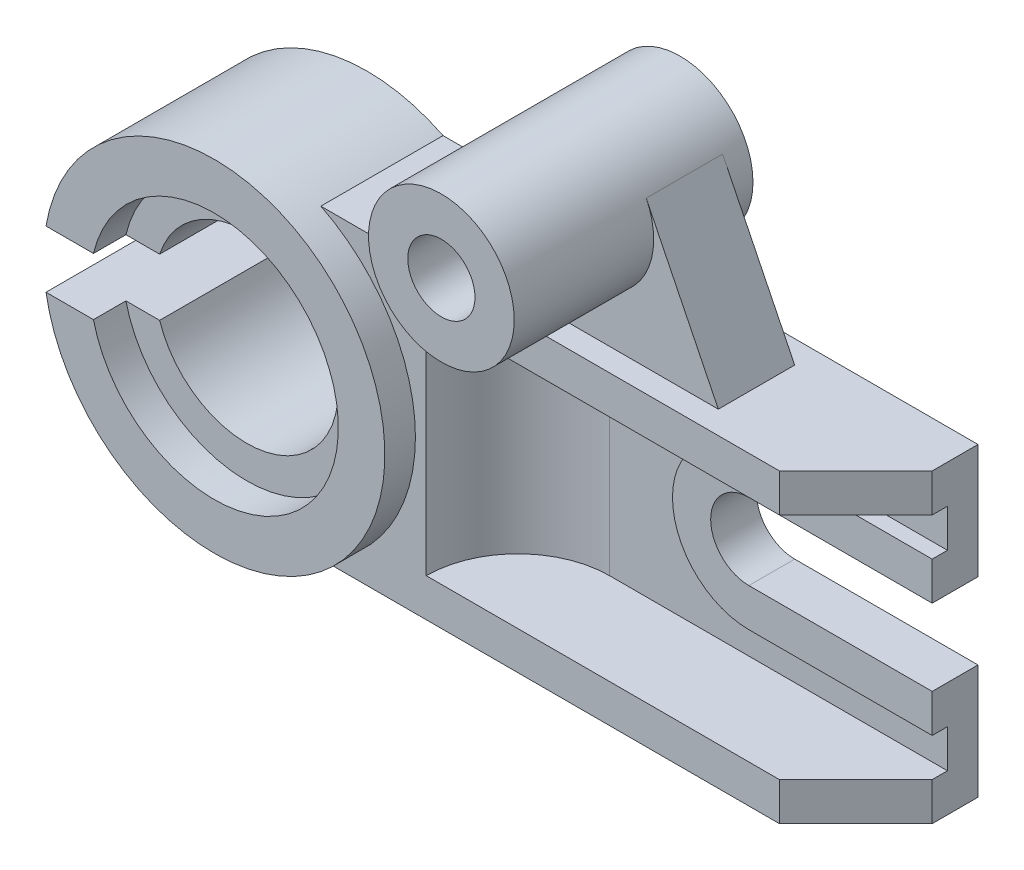
ISO-10303-21;
HEADER;
FILE_DESCRIPTION(('STEP AP214'),'2;1');
FILE_NAME('part.step','',(''),(''),'','','');
FILE_SCHEMA(('AUTOMOTIVE_DESIGN { 1 0 10303 214 1 1 1 1 }'));
ENDSEC;
DATA;
#1=APPLICATION_CONTEXT('core data for automotive mechanical design processes');
#2=APPLICATION_PROTOCOL_DEFINITION('international standard','automotive_design',2000,#1);
#3=PRODUCT_CONTEXT('',#1,'mechanical');
#4=PRODUCT('Part','Part','',(#3));
#5=PRODUCT_RELATED_PRODUCT_CATEGORY('part','',(#4));
#6=PRODUCT_DEFINITION_FORMATION('','',#4);
#7=PRODUCT_DEFINITION_CONTEXT('part definition',#1,'design');
#8=PRODUCT_DEFINITION('design','',#6,#7);
#9=PRODUCT_DEFINITION_SHAPE('','',#8);
#10=(LENGTH_UNIT() NAMED_UNIT(*) SI_UNIT(.MILLI.,.METRE.));
#11=(NAMED_UNIT(*) PLANE_ANGLE_UNIT() SI_UNIT($,.RADIAN.));
#12=(NAMED_UNIT(*) SI_UNIT($,.STERADIAN.) SOLID_ANGLE_UNIT());
#13=UNCERTAINTY_MEASURE_WITH_UNIT(LENGTH_MEASURE(1.E-05),#10,'distance_accuracy_value','');
#14=(GEOMETRIC_REPRESENTATION_CONTEXT(3) GLOBAL_UNCERTAINTY_ASSIGNED_CONTEXT((#13)) GLOBAL_UNIT_ASSIGNED_CONTEXT((#10,
#11,#12)) REPRESENTATION_CONTEXT('',''));
#15=CARTESIAN_POINT('',(0.,0.,0.));
#16=DIRECTION('',(0.,0.,1.));
#17=DIRECTION('',(1.,0.,0.));
#18=AXIS2_PLACEMENT_3D('',#15,#16,#17);
#19=CARTESIAN_POINT('',(4000.,1000.,800.));
#20=DIRECTION('',(-1.,0.,0.));
#21=DIRECTION('',(0.,0.,1.));
#22=AXIS2_PLACEMENT_3D('',#19,#20,#21);
#23=PLANE('',#22);
#24=DIRECTION('',(0.,0.,-1.));
#25=VECTOR('',#24,1.);
#26=CARTESIAN_POINT('',(4000.,1000.,800.));
#27=LINE('',#26,#25);
#28=CARTESIAN_POINT('',(4000.,1000.,299.999999999998));
#29=VERTEX_POINT('',#28);
#30=CARTESIAN_POINT('',(4000.,1000.,0.));
#31=VERTEX_POINT('',#30);
#32=EDGE_CURVE('E361',#29,#31,#27,.T.);
#33=ORIENTED_EDGE('',*,*,#32,.F.);
#34=DIRECTION('',(0.,-1.,0.));
#35=VECTOR('',#34,1.);
#36=CARTESIAN_POINT('',(4000.,750.,299.999999999998));
#37=LINE('',#36,#35);
#38=CARTESIAN_POINT('',(4000.,750.,299.999999999998));
#39=VERTEX_POINT('',#38);
#40=EDGE_CURVE('E430',#29,#39,#37,.T.);
#41=ORIENTED_EDGE('',*,*,#40,.T.);
#42=DIRECTION('',(0.,0.,1.));
#43=VECTOR('',#42,1.);
#44=CARTESIAN_POINT('',(4000.,750.,200.));
#45=LINE('',#44,#43);
#46=CARTESIAN_POINT('',(4000.,750.,200.));
#47=VERTEX_POINT('',#46);
#48=EDGE_CURVE('E335',#47,#39,#45,.T.);
#49=ORIENTED_EDGE('',*,*,#48,.F.);
#50=DIRECTION('',(0.,1.,0.));
#51=VECTOR('',#50,1.);
#52=CARTESIAN_POINT('',(4000.,750.,200.));
#53=LINE('',#52,#51);
#54=CARTESIAN_POINT('',(4000.,500.,200.));
#55=VERTEX_POINT('',#54);
#56=EDGE_CURVE('E320',#55,#47,#53,.T.);
#57=ORIENTED_EDGE('',*,*,#56,.F.);
#58=DIRECTION('',(0.,0.,-1.));
#59=VECTOR('',#58,1.);
#60=CARTESIAN_POINT('',(4000.,500.,300.));
#61=LINE('',#60,#59);
#62=CARTESIAN_POINT('',(4000.,500.,300.));
#63=VERTEX_POINT('',#62);
#64=EDGE_CURVE('E310',#63,#55,#61,.T.);
#65=ORIENTED_EDGE('',*,*,#64,.F.);
#66=DIRECTION('',(0.,1.,0.));
#67=VECTOR('',#66,1.);
#68=CARTESIAN_POINT('',(4000.,500.,300.));
#69=LINE('',#68,#67);
#70=CARTESIAN_POINT('',(4000.,250.,300.));
#71=VERTEX_POINT('',#70);
#72=EDGE_CURVE('E291',#71,#63,#69,.T.);
#73=ORIENTED_EDGE('',*,*,#72,.F.);
#74=DIRECTION('',(0.,0.,1.));
#75=VECTOR('',#74,1.);
#76=CARTESIAN_POINT('',(4000.,250.,0.));
#77=LINE('',#76,#75);
#78=CARTESIAN_POINT('',(4000.,250.,0.));
#79=VERTEX_POINT('',#78);
#80=EDGE_CURVE('E278',#79,#71,#77,.T.);
#81=ORIENTED_EDGE('',*,*,#80,.F.);
#82=DIRECTION('',(0.,1.,0.));
#83=VECTOR('',#82,1.);
#84=CARTESIAN_POINT('',(4000.,1000.,0.));
#85=LINE('',#84,#83);
#86=EDGE_CURVE('E334',#79,#31,#85,.T.);
#87=ORIENTED_EDGE('',*,*,#86,.T.);
#88=EDGE_LOOP('',(#33,#41,#49,#57,#65,#73,#81,#87));
#89=FACE_BOUND('',#88,.T.);
#90=ADVANCED_FACE('F41',(#89),#23,.F.);
#91=CARTESIAN_POINT('',(0.,0.,200.));
#92=DIRECTION('',(0.,0.,1.));
#93=DIRECTION('',(1.,0.,0.));
#94=AXIS2_PLACEMENT_3D('',#91,#92,#93);
#95=PLANE('',#94);
#96=CARTESIAN_POINT('',(4000.,-750.,200.));
#97=VERTEX_POINT('',#96);
#98=CARTESIAN_POINT('',(4000.,-500.,200.));
#99=VERTEX_POINT('',#98);
#100=EDGE_CURVE('E316',#97,#99,#53,.T.);
#101=ORIENTED_EDGE('',*,*,#100,.T.);
#102=DIRECTION('',(1.,0.,0.));
#103=VECTOR('',#102,1.);
#104=CARTESIAN_POINT('',(4000.,-500.,200.));
#105=LINE('',#104,#103);
#106=CARTESIAN_POINT('',(2800.,-500.,200.));
#107=VERTEX_POINT('',#106);
#108=EDGE_CURVE('E305',#107,#99,#105,.T.);
#109=ORIENTED_EDGE('',*,*,#108,.F.);
#110=CARTESIAN_POINT('',(2800.,0.,200.));
#111=DIRECTION('',(0.,0.,1.));
#112=DIRECTION('',(1.,0.,0.));
#113=AXIS2_PLACEMENT_3D('',#110,#111,#112);
#114=CIRCLE('',#113,500.);
#115=CARTESIAN_POINT('',(2800.,500.,200.));
#116=VERTEX_POINT('',#115);
#117=EDGE_CURVE('E276',#116,#107,#114,.T.);
#118=ORIENTED_EDGE('',*,*,#117,.F.);
#119=DIRECTION('',(-1.,0.,0.));
#120=VECTOR('',#119,1.);
#121=CARTESIAN_POINT('',(2800.,500.,200.));
#122=LINE('',#121,#120);
#123=EDGE_CURVE('E293',#55,#116,#122,.T.);
#124=ORIENTED_EDGE('',*,*,#123,.F.);
#125=ORIENTED_EDGE('',*,*,#56,.T.);
#126=DIRECTION('',(-1.,0.,0.));
#127=VECTOR('',#126,1.);
#128=CARTESIAN_POINT('',(1188.,750.,200.));
#129=LINE('',#128,#127);
#130=CARTESIAN_POINT('',(1788.,750.,200.));
#131=VERTEX_POINT('',#130);
#132=EDGE_CURVE('E325',#47,#131,#129,.T.);
#133=ORIENTED_EDGE('',*,*,#132,.T.);
#134=DIRECTION('',(0.,1.,0.));
#135=VECTOR('',#134,1.);
#136=CARTESIAN_POINT('',(1788.,0.,200.));
#137=LINE('',#136,#135);
#138=CARTESIAN_POINT('',(1788.,-750.,200.));
#139=VERTEX_POINT('',#138);
#140=EDGE_CURVE('E415',#131,#139,#137,.F.);
#141=ORIENTED_EDGE('',*,*,#140,.T.);
#142=DIRECTION('',(1.,0.,0.));
#143=VECTOR('',#142,1.);
#144=CARTESIAN_POINT('',(1188.,-750.,200.));
#145=LINE('',#144,#143);
#146=EDGE_CURVE('E314',#139,#97,#145,.T.);
#147=ORIENTED_EDGE('',*,*,#146,.T.);
#148=EDGE_LOOP('',(#101,#109,#118,#124,#125,#133,#141,#147));
#149=FACE_BOUND('',#148,.T.);
#150=ADVANCED_FACE('F501',(#149),#95,.T.);
#151=CARTESIAN_POINT('',(1788.,750.,800.));
#152=DIRECTION('',(0.,1.,0.));
#153=DIRECTION('',(0.,0.,1.));
#154=AXIS2_PLACEMENT_3D('',#151,#152,#153);
#155=CYLINDRICAL_SURFACE('',#154,600.);
#156=DIRECTION('',(0.,-1.,0.));
#157=VECTOR('',#156,1.);
#158=CARTESIAN_POINT('',(1188.,750.,800.));
#159=LINE('',#158,#157);
#160=CARTESIAN_POINT('',(1188.,750.,800.));
#161=VERTEX_POINT('',#160);
#162=CARTESIAN_POINT('',(1188.,-750.,800.));
#163=VERTEX_POINT('',#162);
#164=EDGE_CURVE('E313',#161,#163,#159,.T.);
#165=ORIENTED_EDGE('',*,*,#164,.T.);
#166=CARTESIAN_POINT('',(1788.,-750.,800.));
#167=DIRECTION('',(0.,-1.,0.));
#168=DIRECTION('',(0.,0.,-1.));
#169=AXIS2_PLACEMENT_3D('',#166,#167,#168);
#170=CIRCLE('',#169,600.);
#171=EDGE_CURVE('E416',#139,#163,#170,.F.);
#172=ORIENTED_EDGE('',*,*,#171,.F.);
#173=ORIENTED_EDGE('',*,*,#140,.F.);
#174=CARTESIAN_POINT('',(1788.,750.,800.));
#175=DIRECTION('',(0.,1.,0.));
#176=DIRECTION('',(0.,0.,1.));
#177=AXIS2_PLACEMENT_3D('',#174,#175,#176);
#178=CIRCLE('',#177,600.);
#179=EDGE_CURVE('E419',#161,#131,#178,.F.);
#180=ORIENTED_EDGE('',*,*,#179,.F.);
#181=EDGE_LOOP('',(#165,#172,#173,#180));
#182=FACE_BOUND('',#181,.T.);
#183=ADVANCED_FACE('F458',(#182),#155,.F.);
#184=CARTESIAN_POINT('',(0.,0.,1000.));
#185=DIRECTION('',(0.,0.,-1.));
#186=DIRECTION('',(-1.,0.,0.));
#187=AXIS2_PLACEMENT_3D('',#184,#185,#186);
#188=CYLINDRICAL_SURFACE('',#187,1117.13);
#189=DIRECTION('',(0.,0.,-1.));
#190=VECTOR('',#189,1.);
#191=CARTESIAN_POINT('',(497.975337642338,1000.,800.));
#192=LINE('',#191,#190);
#193=CARTESIAN_POINT('',(497.975337642338,1000.,800.));
#194=VERTEX_POINT('',#193);
#195=CARTESIAN_POINT('',(497.975337642338,1000.,0.));
#196=VERTEX_POINT('',#195);
#197=EDGE_CURVE('E359',#194,#196,#192,.T.);
#198=ORIENTED_EDGE('',*,*,#197,.T.);
#199=CARTESIAN_POINT('',(0.,0.,0.));
#200=DIRECTION('',(0.,0.,1.));
#201=DIRECTION('',(1.,0.,0.));
#202=AXIS2_PLACEMENT_3D('',#199,#200,#201);
#203=CIRCLE('',#202,1117.13);
#204=CARTESIAN_POINT('',(-1101.28251911124,187.5,0.));
#205=VERTEX_POINT('',#204);
#206=EDGE_CURVE('E402',#196,#205,#203,.T.);
#207=ORIENTED_EDGE('',*,*,#206,.T.);
#208=DIRECTION('',(0.,0.,-1.));
#209=VECTOR('',#208,1.);
#210=CARTESIAN_POINT('',(-1101.28251911124,187.5,1000.));
#211=LINE('',#210,#209);
#212=CARTESIAN_POINT('',(-1101.28251911124,187.5,1000.));
#213=VERTEX_POINT('',#212);
#214=EDGE_CURVE('E389',#205,#213,#211,.F.);
#215=ORIENTED_EDGE('',*,*,#214,.T.);
#216=CARTESIAN_POINT('',(0.,0.,1000.));
#217=DIRECTION('',(0.,0.,1.));
#218=DIRECTION('',(1.,0.,0.));
#219=AXIS2_PLACEMENT_3D('',#216,#217,#218);
#220=CIRCLE('',#219,1117.13);
#221=CARTESIAN_POINT('',(-1101.28251911124,-187.5,1000.));
#222=VERTEX_POINT('',#221);
#223=EDGE_CURVE('E404',#222,#213,#220,.T.);
#224=ORIENTED_EDGE('',*,*,#223,.F.);
#225=DIRECTION('',(0.,0.,-1.));
#226=VECTOR('',#225,1.);
#227=CARTESIAN_POINT('',(-1101.28251911124,-187.5,1000.));
#228=LINE('',#227,#226);
#229=CARTESIAN_POINT('',(-1101.28251911124,-187.5,0.));
#230=VERTEX_POINT('',#229);
#231=EDGE_CURVE('E379',#222,#230,#228,.T.);
#232=ORIENTED_EDGE('',*,*,#231,.T.);
#233=CARTESIAN_POINT('',(497.975337642337,-1000.,0.));
#234=VERTEX_POINT('',#233);
#235=EDGE_CURVE('E409',#230,#234,#203,.T.);
#236=ORIENTED_EDGE('',*,*,#235,.T.);
#237=DIRECTION('',(0.,0.,-1.));
#238=VECTOR('',#237,1.);
#239=CARTESIAN_POINT('',(497.975337642338,-1000.,800.));
#240=LINE('',#239,#238);
#241=CARTESIAN_POINT('',(497.975337642338,-1000.,800.));
#242=VERTEX_POINT('',#241);
#243=EDGE_CURVE('E357',#242,#234,#240,.T.);
#244=ORIENTED_EDGE('',*,*,#243,.F.);
#245=CARTESIAN_POINT('',(0.,0.,800.));
#246=DIRECTION('',(0.,0.,-1.));
#247=DIRECTION('',(1.,0.,0.));
#248=AXIS2_PLACEMENT_3D('',#245,#246,#247);
#249=CIRCLE('',#248,1117.13);
#250=EDGE_CURVE('E338',#194,#242,#249,.T.);
#251=ORIENTED_EDGE('',*,*,#250,.F.);
#252=EDGE_LOOP('',(#198,#207,#215,#224,#232,#236,#244,#251));
#253=FACE_BOUND('',#252,.T.);
#254=ADVANCED_FACE('F481',(#253),#188,.T.);
#255=CARTESIAN_POINT('',(0.,0.,1000.));
#256=DIRECTION('',(0.,0.,1.));
#257=DIRECTION('',(1.,0.,0.));
#258=AXIS2_PLACEMENT_3D('',#255,#256,#257);
#259=PLANE('',#258);
#260=DIRECTION('',(-1.,0.,0.));
#261=VECTOR('',#260,1.);
#262=CARTESIAN_POINT('',(-1240.32055513707,187.5,1000.));
#263=LINE('',#262,#261);
#264=CARTESIAN_POINT('',(-790.569415042095,187.5,1000.));
#265=VERTEX_POINT('',#264);
#266=EDGE_CURVE('E369',#265,#213,#263,.T.);
#267=ORIENTED_EDGE('',*,*,#266,.F.);
#268=CARTESIAN_POINT('',(0.,0.,1000.));
#269=DIRECTION('',(0.,0.,1.));
#270=DIRECTION('',(1.,0.,0.));
#271=AXIS2_PLACEMENT_3D('',#268,#269,#270);
#272=CIRCLE('',#271,812.5);
#273=CARTESIAN_POINT('',(-790.569415042095,-187.5,1000.));
#274=VERTEX_POINT('',#273);
#275=EDGE_CURVE('E395',#274,#265,#272,.T.);
#276=ORIENTED_EDGE('',*,*,#275,.F.);
#277=DIRECTION('',(1.,0.,0.));
#278=VECTOR('',#277,1.);
#279=CARTESIAN_POINT('',(-1240.32055513707,-187.5,1000.));
#280=LINE('',#279,#278);
#281=EDGE_CURVE('E362',#222,#274,#280,.T.);
#282=ORIENTED_EDGE('',*,*,#281,.F.);
#283=ORIENTED_EDGE('',*,*,#223,.T.);
#284=EDGE_LOOP('',(#267,#276,#282,#283));
#285=FACE_BOUND('',#284,.T.);
#286=ADVANCED_FACE('F563',(#285),#259,.T.);
#287=CARTESIAN_POINT('',(0.,0.,0.));
#288=DIRECTION('',(0.,0.,1.));
#289=DIRECTION('',(1.,0.,0.));
#290=AXIS2_PLACEMENT_3D('',#287,#288,#289);
#291=PLANE('',#290);
#292=ORIENTED_EDGE('',*,*,#86,.F.);
#293=DIRECTION('',(-1.,0.,0.));
#294=VECTOR('',#293,1.);
#295=CARTESIAN_POINT('',(2800.,250.,0.));
#296=LINE('',#295,#294);
#297=CARTESIAN_POINT('',(2800.,250.,0.));
#298=VERTEX_POINT('',#297);
#299=EDGE_CURVE('E266',#79,#298,#296,.T.);
#300=ORIENTED_EDGE('',*,*,#299,.T.);
#301=CARTESIAN_POINT('',(2800.,0.,0.));
#302=DIRECTION('',(0.,0.,1.));
#303=DIRECTION('',(1.,0.,0.));
#304=AXIS2_PLACEMENT_3D('',#301,#302,#303);
#305=CIRCLE('',#304,250.);
#306=CARTESIAN_POINT('',(2800.,-250.,0.));
#307=VERTEX_POINT('',#306);
#308=EDGE_CURVE('E261',#298,#307,#305,.T.);
#309=ORIENTED_EDGE('',*,*,#308,.T.);
#310=DIRECTION('',(1.,0.,0.));
#311=VECTOR('',#310,1.);
#312=CARTESIAN_POINT('',(4000.,-250.,0.));
#313=LINE('',#312,#311);
#314=CARTESIAN_POINT('',(4000.,-250.,0.));
#315=VERTEX_POINT('',#314);
#316=EDGE_CURVE('E263',#307,#315,#313,.T.);
#317=ORIENTED_EDGE('',*,*,#316,.T.);
#318=CARTESIAN_POINT('',(4000.,-1000.,0.));
#319=VERTEX_POINT('',#318);
#320=EDGE_CURVE('E349',#319,#315,#85,.T.);
#321=ORIENTED_EDGE('',*,*,#320,.F.);
#322=DIRECTION('',(1.,0.,0.));
#323=VECTOR('',#322,1.);
#324=CARTESIAN_POINT('',(497.975337642338,-1000.,0.));
#325=LINE('',#324,#323);
#326=EDGE_CURVE('E342',#234,#319,#325,.T.);
#327=ORIENTED_EDGE('',*,*,#326,.F.);
#328=ORIENTED_EDGE('',*,*,#235,.F.);
#329=DIRECTION('',(1.,0.,0.));
#330=VECTOR('',#329,1.);
#331=CARTESIAN_POINT('',(-1240.32055513707,-187.5,0.));
#332=LINE('',#331,#330);
#333=CARTESIAN_POINT('',(-569.9506557589,-187.5,0.));
#334=VERTEX_POINT('',#333);
#335=EDGE_CURVE('E366',#230,#334,#332,.T.);
#336=ORIENTED_EDGE('',*,*,#335,.T.);
#337=CARTESIAN_POINT('',(0.,0.,0.));
#338=DIRECTION('',(0.,0.,1.));
#339=DIRECTION('',(1.,0.,0.));
#340=AXIS2_PLACEMENT_3D('',#337,#338,#339);
#341=CIRCLE('',#340,600.);
#342=CARTESIAN_POINT('',(-569.9506557589,187.5,0.));
#343=VERTEX_POINT('',#342);
#344=EDGE_CURVE('E392',#334,#343,#341,.T.);
#345=ORIENTED_EDGE('',*,*,#344,.T.);
#346=DIRECTION('',(-1.,0.,0.));
#347=VECTOR('',#346,1.);
#348=CARTESIAN_POINT('',(-1240.32055513707,187.5,0.));
#349=LINE('',#348,#347);
#350=EDGE_CURVE('E367',#343,#205,#349,.T.);
#351=ORIENTED_EDGE('',*,*,#350,.T.);
#352=ORIENTED_EDGE('',*,*,#206,.F.);
#353=DIRECTION('',(-1.,0.,0.));
#354=VECTOR('',#353,1.);
#355=CARTESIAN_POINT('',(497.975337642338,1000.,0.));
#356=LINE('',#355,#354);
#357=EDGE_CURVE('E353',#31,#196,#356,.T.);
#358=ORIENTED_EDGE('',*,*,#357,.F.);
#359=EDGE_LOOP('',(#292,#300,#309,#317,#321,#327,#328,#336,#345,#351,#352,#358));
#360=FACE_BOUND('',#359,.T.);
#361=ADVANCED_FACE('F480',(#360),#291,.F.);
#362=CARTESIAN_POINT('',(0.,0.,787.5));
#363=DIRECTION('',(0.,0.,1.));
#364=DIRECTION('',(1.,0.,0.));
#365=AXIS2_PLACEMENT_3D('',#362,#363,#364);
#366=CYLINDRICAL_SURFACE('',#365,812.5);
#367=ORIENTED_EDGE('',*,*,#275,.T.);
#368=DIRECTION('',(0.,0.,1.));
#369=VECTOR('',#368,1.);
#370=CARTESIAN_POINT('',(-790.569415042095,187.5,787.5));
#371=LINE('',#370,#369);
#372=CARTESIAN_POINT('',(-790.569415042095,187.5,787.5));
#373=VERTEX_POINT('',#372);
#374=EDGE_CURVE('E383',#265,#373,#371,.F.);
#375=ORIENTED_EDGE('',*,*,#374,.T.);
#376=CARTESIAN_POINT('',(0.,0.,787.5));
#377=DIRECTION('',(0.,0.,1.));
#378=DIRECTION('',(1.,0.,0.));
#379=AXIS2_PLACEMENT_3D('',#376,#377,#378);
#380=CIRCLE('',#379,812.5);
#381=CARTESIAN_POINT('',(-790.569415042095,-187.5,787.5));
#382=VERTEX_POINT('',#381);
#383=EDGE_CURVE('E396',#382,#373,#380,.T.);
#384=ORIENTED_EDGE('',*,*,#383,.F.);
#385=DIRECTION('',(0.,0.,1.));
#386=VECTOR('',#385,1.);
#387=CARTESIAN_POINT('',(-790.569415042095,-187.5,787.5));
#388=LINE('',#387,#386);
#389=EDGE_CURVE('E380',#382,#274,#388,.T.);
#390=ORIENTED_EDGE('',*,*,#389,.T.);
#391=EDGE_LOOP('',(#367,#375,#384,#390));
#392=FACE_BOUND('',#391,.T.);
#393=ADVANCED_FACE('F556',(#392),#366,.F.);
#394=CARTESIAN_POINT('',(0.,0.,787.5));
#395=DIRECTION('',(0.,0.,1.));
#396=DIRECTION('',(1.,0.,0.));
#397=AXIS2_PLACEMENT_3D('',#394,#395,#396);
#398=PLANE('',#397);
#399=DIRECTION('',(-1.,0.,0.));
#400=VECTOR('',#399,1.);
#401=CARTESIAN_POINT('',(0.,187.5,787.5));
#402=LINE('',#401,#400);
#403=CARTESIAN_POINT('',(-569.9506557589,187.5,787.5));
#404=VERTEX_POINT('',#403);
#405=EDGE_CURVE('E384',#404,#373,#402,.T.);
#406=ORIENTED_EDGE('',*,*,#405,.F.);
#407=CARTESIAN_POINT('',(0.,0.,787.5));
#408=DIRECTION('',(0.,0.,1.));
#409=DIRECTION('',(1.,0.,0.));
#410=AXIS2_PLACEMENT_3D('',#407,#408,#409);
#411=CIRCLE('',#410,600.);
#412=CARTESIAN_POINT('',(-569.9506557589,-187.5,787.5));
#413=VERTEX_POINT('',#412);
#414=EDGE_CURVE('E391',#413,#404,#411,.T.);
#415=ORIENTED_EDGE('',*,*,#414,.F.);
#416=DIRECTION('',(1.,0.,0.));
#417=VECTOR('',#416,1.);
#418=CARTESIAN_POINT('',(0.,-187.5,787.5));
#419=LINE('',#418,#417);
#420=EDGE_CURVE('E373',#382,#413,#419,.T.);
#421=ORIENTED_EDGE('',*,*,#420,.F.);
#422=ORIENTED_EDGE('',*,*,#383,.T.);
#423=EDGE_LOOP('',(#406,#415,#421,#422));
#424=FACE_BOUND('',#423,.T.);
#425=ADVANCED_FACE('F555',(#424),#398,.T.);
#426=CARTESIAN_POINT('',(0.,0.,0.));
#427=DIRECTION('',(0.,0.,1.));
#428=DIRECTION('',(1.,0.,0.));
#429=AXIS2_PLACEMENT_3D('',#426,#427,#428);
#430=CYLINDRICAL_SURFACE('',#429,600.);
#431=ORIENTED_EDGE('',*,*,#414,.T.);
#432=DIRECTION('',(0.,0.,1.));
#433=VECTOR('',#432,1.);
#434=CARTESIAN_POINT('',(-569.9506557589,187.5,0.));
#435=LINE('',#434,#433);
#436=EDGE_CURVE('E412',#404,#343,#435,.F.);
#437=ORIENTED_EDGE('',*,*,#436,.T.);
#438=ORIENTED_EDGE('',*,*,#344,.F.);
#439=DIRECTION('',(0.,0.,1.));
#440=VECTOR('',#439,1.);
#441=CARTESIAN_POINT('',(-569.9506557589,-187.5,0.));
#442=LINE('',#441,#440);
#443=EDGE_CURVE('E410',#334,#413,#442,.T.);
#444=ORIENTED_EDGE('',*,*,#443,.T.);
#445=EDGE_LOOP('',(#431,#437,#438,#444));
#446=FACE_BOUND('',#445,.T.);
#447=ADVANCED_FACE('F546',(#446),#430,.F.);
#448=CARTESIAN_POINT('',(-1240.32055513707,-187.5,0.));
#449=DIRECTION('',(0.,-1.,0.));
#450=DIRECTION('',(0.,0.,-1.));
#451=AXIS2_PLACEMENT_3D('',#448,#449,#450);
#452=PLANE('',#451);
#453=ORIENTED_EDGE('',*,*,#281,.T.);
#454=ORIENTED_EDGE('',*,*,#389,.F.);
#455=ORIENTED_EDGE('',*,*,#420,.T.);
#456=ORIENTED_EDGE('',*,*,#443,.F.);
#457=ORIENTED_EDGE('',*,*,#335,.F.);
#458=ORIENTED_EDGE('',*,*,#231,.F.);
#459=EDGE_LOOP('',(#453,#454,#455,#456,#457,#458));
#460=FACE_BOUND('',#459,.T.);
#461=ADVANCED_FACE('F542',(#460),#452,.F.);
#462=CARTESIAN_POINT('',(-1240.32055513707,187.5,0.));
#463=DIRECTION('',(0.,1.,0.));
#464=DIRECTION('',(0.,0.,1.));
#465=AXIS2_PLACEMENT_3D('',#462,#463,#464);
#466=PLANE('',#465);
#467=ORIENTED_EDGE('',*,*,#350,.F.);
#468=ORIENTED_EDGE('',*,*,#436,.F.);
#469=ORIENTED_EDGE('',*,*,#405,.T.);
#470=ORIENTED_EDGE('',*,*,#374,.F.);
#471=ORIENTED_EDGE('',*,*,#266,.T.);
#472=ORIENTED_EDGE('',*,*,#214,.F.);
#473=EDGE_LOOP('',(#467,#468,#469,#470,#471,#472));
#474=FACE_BOUND('',#473,.T.);
#475=ADVANCED_FACE('F537',(#474),#466,.F.);
#476=DIRECTION('',(0.,0.,1.));
#477=VECTOR('',#476,1.);
#478=CARTESIAN_POINT('',(4000.,-750.,200.));
#479=LINE('',#478,#477);
#480=CARTESIAN_POINT('',(4000.,-750.,299.999999999998));
#481=VERTEX_POINT('',#480);
#482=EDGE_CURVE('E323',#97,#481,#479,.T.);
#483=ORIENTED_EDGE('',*,*,#482,.T.);
#484=DIRECTION('',(0.,-1.,0.));
#485=VECTOR('',#484,1.);
#486=CARTESIAN_POINT('',(4000.,-1000.,299.999999999998));
#487=LINE('',#486,#485);
#488=CARTESIAN_POINT('',(4000.,-1000.,299.999999999998));
#489=VERTEX_POINT('',#488);
#490=EDGE_CURVE('E49',#481,#489,#487,.T.);
#491=ORIENTED_EDGE('',*,*,#490,.T.);
#492=DIRECTION('',(0.,0.,-1.));
#493=VECTOR('',#492,1.);
#494=CARTESIAN_POINT('',(4000.,-1000.,800.));
#495=LINE('',#494,#493);
#496=EDGE_CURVE('E347',#489,#319,#495,.T.);
#497=ORIENTED_EDGE('',*,*,#496,.T.);
#498=ORIENTED_EDGE('',*,*,#320,.T.);
#499=DIRECTION('',(0.,0.,1.));
#500=VECTOR('',#499,1.);
#501=CARTESIAN_POINT('',(4000.,-250.,0.));
#502=LINE('',#501,#500);
#503=CARTESIAN_POINT('',(4000.,-250.,300.));
#504=VERTEX_POINT('',#503);
#505=EDGE_CURVE('E282',#315,#504,#502,.T.);
#506=ORIENTED_EDGE('',*,*,#505,.T.);
#507=CARTESIAN_POINT('',(4000.,-500.,300.));
#508=VERTEX_POINT('',#507);
#509=EDGE_CURVE('E295',#508,#504,#69,.T.);
#510=ORIENTED_EDGE('',*,*,#509,.F.);
#511=DIRECTION('',(0.,0.,-1.));
#512=VECTOR('',#511,1.);
#513=CARTESIAN_POINT('',(4000.,-500.,300.));
#514=LINE('',#513,#512);
#515=EDGE_CURVE('E307',#508,#99,#514,.T.);
#516=ORIENTED_EDGE('',*,*,#515,.T.);
#517=ORIENTED_EDGE('',*,*,#100,.F.);
#518=EDGE_LOOP('',(#483,#491,#497,#498,#506,#510,#516,#517));
#519=FACE_BOUND('',#518,.T.);
#520=ADVANCED_FACE('F438',(#519),#23,.F.);
#521=CARTESIAN_POINT('',(497.975337642338,1000.,800.));
#522=DIRECTION('',(0.,-1.,0.));
#523=DIRECTION('',(1.,0.,0.));
#524=AXIS2_PLACEMENT_3D('',#521,#522,#523);
#525=PLANE('',#524);
#526=DIRECTION('',(0.,0.,-1.));
#527=VECTOR('',#526,1.);
#528=CARTESIAN_POINT('',(2950.,1000.,650.));
#529=LINE('',#528,#527);
#530=CARTESIAN_POINT('',(2950.,1000.,650.));
#531=VERTEX_POINT('',#530);
#532=CARTESIAN_POINT('',(2950.,1000.,150.));
#533=VERTEX_POINT('',#532);
#534=EDGE_CURVE('E60',#531,#533,#529,.T.);
#535=ORIENTED_EDGE('',*,*,#534,.F.);
#536=DIRECTION('',(1.,0.,0.));
#537=VECTOR('',#536,1.);
#538=CARTESIAN_POINT('',(1150.,1000.,650.));
#539=LINE('',#538,#537);
#540=CARTESIAN_POINT('',(1150.,1000.,650.));
#541=VERTEX_POINT('',#540);
#542=EDGE_CURVE('E62',#541,#531,#539,.T.);
#543=ORIENTED_EDGE('',*,*,#542,.F.);
#544=DIRECTION('',(0.,0.,-1.));
#545=VECTOR('',#544,1.);
#546=CARTESIAN_POINT('',(1150.,1000.,650.));
#547=LINE('',#546,#545);
#548=CARTESIAN_POINT('',(1150.,1000.,150.));
#549=VERTEX_POINT('',#548);
#550=EDGE_CURVE('E243',#541,#549,#547,.T.);
#551=ORIENTED_EDGE('',*,*,#550,.T.);
#552=DIRECTION('',(1.,0.,0.));
#553=VECTOR('',#552,1.);
#554=CARTESIAN_POINT('',(1150.,1000.,150.));
#555=LINE('',#554,#553);
#556=EDGE_CURVE('E233',#549,#533,#555,.T.);
#557=ORIENTED_EDGE('',*,*,#556,.T.);
#558=EDGE_LOOP('',(#535,#543,#551,#557));
#559=FACE_BOUND('',#558,.T.);
#560=DIRECTION('',(-1.,0.,0.));
#561=VECTOR('',#560,1.);
#562=CARTESIAN_POINT('',(497.975337642338,1000.,800.));
#563=LINE('',#562,#561);
#564=CARTESIAN_POINT('',(3500.,1000.,800.));
#565=VERTEX_POINT('',#564);
#566=EDGE_CURVE('E336',#565,#194,#563,.T.);
#567=ORIENTED_EDGE('',*,*,#566,.F.);
#568=DIRECTION('',(0.707106781186546,0.,-0.707106781186549));
#569=VECTOR('',#568,1.);
#570=CARTESIAN_POINT('',(3500.,1000.,800.));
#571=LINE('',#570,#569);
#572=EDGE_CURVE('E424',#565,#29,#571,.T.);
#573=ORIENTED_EDGE('',*,*,#572,.T.);
#574=ORIENTED_EDGE('',*,*,#32,.T.);
#575=ORIENTED_EDGE('',*,*,#357,.T.);
#576=ORIENTED_EDGE('',*,*,#197,.F.);
#577=EDGE_LOOP('',(#567,#573,#574,#575,#576));
#578=FACE_BOUND('',#577,.T.);
#579=ADVANCED_FACE('F468',(#559,#578),#525,.F.);
#580=CARTESIAN_POINT('',(497.975337642338,-1000.,800.));
#581=DIRECTION('',(0.,1.,0.));
#582=DIRECTION('',(0.,0.,1.));
#583=AXIS2_PLACEMENT_3D('',#580,#581,#582);
#584=PLANE('',#583);
#585=ORIENTED_EDGE('',*,*,#496,.F.);
#586=DIRECTION('',(-0.707106781186546,0.,0.707106781186549));
#587=VECTOR('',#586,1.);
#588=CARTESIAN_POINT('',(3500.,-1000.,800.));
#589=LINE('',#588,#587);
#590=CARTESIAN_POINT('',(3500.,-1000.,800.));
#591=VERTEX_POINT('',#590);
#592=EDGE_CURVE('E11',#489,#591,#589,.T.);
#593=ORIENTED_EDGE('',*,*,#592,.T.);
#594=DIRECTION('',(1.,0.,0.));
#595=VECTOR('',#594,1.);
#596=CARTESIAN_POINT('',(497.975337642338,-1000.,800.));
#597=LINE('',#596,#595);
#598=EDGE_CURVE('E341',#242,#591,#597,.T.);
#599=ORIENTED_EDGE('',*,*,#598,.F.);
#600=ORIENTED_EDGE('',*,*,#243,.T.);
#601=ORIENTED_EDGE('',*,*,#326,.T.);
#602=EDGE_LOOP('',(#585,#593,#599,#600,#601));
#603=FACE_BOUND('',#602,.T.);
#604=ADVANCED_FACE('F443',(#603),#584,.F.);
#605=CARTESIAN_POINT('',(0.,0.,800.));
#606=DIRECTION('',(0.,0.,1.));
#607=DIRECTION('',(1.,0.,0.));
#608=AXIS2_PLACEMENT_3D('',#605,#606,#607);
#609=PLANE('',#608);
#610=ORIENTED_EDGE('',*,*,#598,.T.);
#611=DIRECTION('',(0.,1.,0.));
#612=VECTOR('',#611,1.);
#613=CARTESIAN_POINT('',(3500.,-750.,800.));
#614=LINE('',#613,#612);
#615=CARTESIAN_POINT('',(3500.,-750.,800.));
#616=VERTEX_POINT('',#615);
#617=EDGE_CURVE('E431',#591,#616,#614,.T.);
#618=ORIENTED_EDGE('',*,*,#617,.T.);
#619=DIRECTION('',(1.,0.,0.));
#620=VECTOR('',#619,1.);
#621=CARTESIAN_POINT('',(1188.,-750.,800.));
#622=LINE('',#621,#620);
#623=EDGE_CURVE('E329',#163,#616,#622,.T.);
#624=ORIENTED_EDGE('',*,*,#623,.F.);
#625=ORIENTED_EDGE('',*,*,#164,.F.);
#626=DIRECTION('',(-1.,0.,0.));
#627=VECTOR('',#626,1.);
#628=CARTESIAN_POINT('',(1188.,750.,800.));
#629=LINE('',#628,#627);
#630=CARTESIAN_POINT('',(3500.,750.,800.));
#631=VERTEX_POINT('',#630);
#632=EDGE_CURVE('E319',#631,#161,#629,.T.);
#633=ORIENTED_EDGE('',*,*,#632,.F.);
#634=DIRECTION('',(0.,1.,0.));
#635=VECTOR('',#634,1.);
#636=CARTESIAN_POINT('',(3500.,1000.,800.));
#637=LINE('',#636,#635);
#638=EDGE_CURVE('E422',#631,#565,#637,.T.);
#639=ORIENTED_EDGE('',*,*,#638,.T.);
#640=ORIENTED_EDGE('',*,*,#566,.T.);
#641=ORIENTED_EDGE('',*,*,#250,.T.);
#642=EDGE_LOOP('',(#610,#618,#624,#625,#633,#639,#640,#641));
#643=FACE_BOUND('',#642,.T.);
#644=ADVANCED_FACE('F452',(#643),#609,.T.);
#645=CARTESIAN_POINT('',(1188.,750.,200.));
#646=DIRECTION('',(0.,1.,0.));
#647=DIRECTION('',(0.,0.,1.));
#648=AXIS2_PLACEMENT_3D('',#645,#646,#647);
#649=PLANE('',#648);
#650=ORIENTED_EDGE('',*,*,#48,.T.);
#651=DIRECTION('',(-0.707106781186546,0.,0.707106781186549));
#652=VECTOR('',#651,1.);
#653=CARTESIAN_POINT('',(3500.,750.,800.));
#654=LINE('',#653,#652);
#655=EDGE_CURVE('E429',#39,#631,#654,.T.);
#656=ORIENTED_EDGE('',*,*,#655,.T.);
#657=ORIENTED_EDGE('',*,*,#632,.T.);
#658=ORIENTED_EDGE('',*,*,#179,.T.);
#659=ORIENTED_EDGE('',*,*,#132,.F.);
#660=EDGE_LOOP('',(#650,#656,#657,#658,#659));
#661=FACE_BOUND('',#660,.T.);
#662=ADVANCED_FACE('F506',(#661),#649,.F.);
#663=CARTESIAN_POINT('',(1188.,-750.,200.));
#664=DIRECTION('',(0.,-1.,0.));
#665=DIRECTION('',(0.,0.,-1.));
#666=AXIS2_PLACEMENT_3D('',#663,#664,#665);
#667=PLANE('',#666);
#668=ORIENTED_EDGE('',*,*,#623,.T.);
#669=DIRECTION('',(0.707106781186546,0.,-0.707106781186549));
#670=VECTOR('',#669,1.);
#671=CARTESIAN_POINT('',(3500.,-750.,800.));
#672=LINE('',#671,#670);
#673=EDGE_CURVE('E432',#616,#481,#672,.T.);
#674=ORIENTED_EDGE('',*,*,#673,.T.);
#675=ORIENTED_EDGE('',*,*,#482,.F.);
#676=ORIENTED_EDGE('',*,*,#146,.F.);
#677=ORIENTED_EDGE('',*,*,#171,.T.);
#678=EDGE_LOOP('',(#668,#674,#675,#676,#677));
#679=FACE_BOUND('',#678,.T.);
#680=ADVANCED_FACE('F451',(#679),#667,.F.);
#681=CARTESIAN_POINT('',(2800.,0.,300.));
#682=DIRECTION('',(0.,0.,-1.));
#683=DIRECTION('',(-1.,0.,0.));
#684=AXIS2_PLACEMENT_3D('',#681,#682,#683);
#685=CYLINDRICAL_SURFACE('',#684,500.);
#686=ORIENTED_EDGE('',*,*,#117,.T.);
#687=DIRECTION('',(0.,0.,-1.));
#688=VECTOR('',#687,1.);
#689=CARTESIAN_POINT('',(2800.,-500.,300.));
#690=LINE('',#689,#688);
#691=CARTESIAN_POINT('',(2800.,-500.,300.));
#692=VERTEX_POINT('',#691);
#693=EDGE_CURVE('E315',#692,#107,#690,.T.);
#694=ORIENTED_EDGE('',*,*,#693,.F.);
#695=CARTESIAN_POINT('',(2800.,0.,300.));
#696=DIRECTION('',(0.,0.,1.));
#697=DIRECTION('',(1.,0.,0.));
#698=AXIS2_PLACEMENT_3D('',#695,#696,#697);
#699=CIRCLE('',#698,500.);
#700=CARTESIAN_POINT('',(2800.,500.,300.));
#701=VERTEX_POINT('',#700);
#702=EDGE_CURVE('E290',#701,#692,#699,.T.);
#703=ORIENTED_EDGE('',*,*,#702,.F.);
#704=DIRECTION('',(0.,0.,-1.));
#705=VECTOR('',#704,1.);
#706=CARTESIAN_POINT('',(2800.,500.,300.));
#707=LINE('',#706,#705);
#708=EDGE_CURVE('E299',#701,#116,#707,.T.);
#709=ORIENTED_EDGE('',*,*,#708,.T.);
#710=EDGE_LOOP('',(#686,#694,#703,#709));
#711=FACE_BOUND('',#710,.T.);
#712=ADVANCED_FACE('F590',(#711),#685,.T.);
#713=CARTESIAN_POINT('',(4000.,-500.,300.));
#714=DIRECTION('',(0.,1.,0.));
#715=DIRECTION('',(0.,0.,1.));
#716=AXIS2_PLACEMENT_3D('',#713,#714,#715);
#717=PLANE('',#716);
#718=ORIENTED_EDGE('',*,*,#108,.T.);
#719=ORIENTED_EDGE('',*,*,#515,.F.);
#720=DIRECTION('',(1.,0.,0.));
#721=VECTOR('',#720,1.);
#722=CARTESIAN_POINT('',(4000.,-500.,300.));
#723=LINE('',#722,#721);
#724=EDGE_CURVE('E289',#692,#508,#723,.T.);
#725=ORIENTED_EDGE('',*,*,#724,.F.);
#726=ORIENTED_EDGE('',*,*,#693,.T.);
#727=EDGE_LOOP('',(#718,#719,#725,#726));
#728=FACE_BOUND('',#727,.T.);
#729=ADVANCED_FACE('F498',(#728),#717,.F.);
#730=CARTESIAN_POINT('',(2800.,500.,300.));
#731=DIRECTION('',(0.,-1.,0.));
#732=DIRECTION('',(1.,0.,0.));
#733=AXIS2_PLACEMENT_3D('',#730,#731,#732);
#734=PLANE('',#733);
#735=ORIENTED_EDGE('',*,*,#123,.T.);
#736=ORIENTED_EDGE('',*,*,#708,.F.);
#737=DIRECTION('',(-1.,0.,0.));
#738=VECTOR('',#737,1.);
#739=CARTESIAN_POINT('',(2800.,500.,300.));
#740=LINE('',#739,#738);
#741=EDGE_CURVE('E300',#63,#701,#740,.T.);
#742=ORIENTED_EDGE('',*,*,#741,.F.);
#743=ORIENTED_EDGE('',*,*,#64,.T.);
#744=EDGE_LOOP('',(#735,#736,#742,#743));
#745=FACE_BOUND('',#744,.T.);
#746=ADVANCED_FACE('F512',(#745),#734,.F.);
#747=CARTESIAN_POINT('',(2800.,0.,300.));
#748=DIRECTION('',(0.,0.,1.));
#749=DIRECTION('',(1.,0.,0.));
#750=AXIS2_PLACEMENT_3D('',#747,#748,#749);
#751=PLANE('',#750);
#752=DIRECTION('',(-1.,0.,0.));
#753=VECTOR('',#752,1.);
#754=CARTESIAN_POINT('',(2800.,250.,300.));
#755=LINE('',#754,#753);
#756=CARTESIAN_POINT('',(2800.,250.,300.));
#757=VERTEX_POINT('',#756);
#758=EDGE_CURVE('E265',#71,#757,#755,.T.);
#759=ORIENTED_EDGE('',*,*,#758,.F.);
#760=ORIENTED_EDGE('',*,*,#72,.T.);
#761=ORIENTED_EDGE('',*,*,#741,.T.);
#762=ORIENTED_EDGE('',*,*,#702,.T.);
#763=ORIENTED_EDGE('',*,*,#724,.T.);
#764=ORIENTED_EDGE('',*,*,#509,.T.);
#765=DIRECTION('',(1.,0.,0.));
#766=VECTOR('',#765,1.);
#767=CARTESIAN_POINT('',(4000.,-250.,300.));
#768=LINE('',#767,#766);
#769=CARTESIAN_POINT('',(2800.,-250.,300.));
#770=VERTEX_POINT('',#769);
#771=EDGE_CURVE('E271',#770,#504,#768,.T.);
#772=ORIENTED_EDGE('',*,*,#771,.F.);
#773=CARTESIAN_POINT('',(2800.,0.,300.));
#774=DIRECTION('',(0.,0.,1.));
#775=DIRECTION('',(1.,0.,0.));
#776=AXIS2_PLACEMENT_3D('',#773,#774,#775);
#777=CIRCLE('',#776,250.);
#778=EDGE_CURVE('E258',#757,#770,#777,.T.);
#779=ORIENTED_EDGE('',*,*,#778,.F.);
#780=EDGE_LOOP('',(#759,#760,#761,#762,#763,#764,#772,#779));
#781=FACE_BOUND('',#780,.T.);
#782=ADVANCED_FACE('F495',(#781),#751,.T.);
#783=CARTESIAN_POINT('',(2800.,0.,0.));
#784=DIRECTION('',(0.,0.,1.));
#785=DIRECTION('',(1.,0.,0.));
#786=AXIS2_PLACEMENT_3D('',#783,#784,#785);
#787=CYLINDRICAL_SURFACE('',#786,250.);
#788=ORIENTED_EDGE('',*,*,#778,.T.);
#789=DIRECTION('',(0.,0.,1.));
#790=VECTOR('',#789,1.);
#791=CARTESIAN_POINT('',(2800.,-250.,0.));
#792=LINE('',#791,#790);
#793=EDGE_CURVE('E272',#307,#770,#792,.T.);
#794=ORIENTED_EDGE('',*,*,#793,.F.);
#795=ORIENTED_EDGE('',*,*,#308,.F.);
#796=DIRECTION('',(0.,0.,1.));
#797=VECTOR('',#796,1.);
#798=CARTESIAN_POINT('',(2800.,250.,0.));
#799=LINE('',#798,#797);
#800=EDGE_CURVE('E280',#298,#757,#799,.T.);
#801=ORIENTED_EDGE('',*,*,#800,.T.);
#802=EDGE_LOOP('',(#788,#794,#795,#801));
#803=FACE_BOUND('',#802,.T.);
#804=ADVANCED_FACE('F517',(#803),#787,.F.);
#805=CARTESIAN_POINT('',(2800.,250.,0.));
#806=DIRECTION('',(0.,1.,0.));
#807=DIRECTION('',(-1.,0.,0.));
#808=AXIS2_PLACEMENT_3D('',#805,#806,#807);
#809=PLANE('',#808);
#810=ORIENTED_EDGE('',*,*,#758,.T.);
#811=ORIENTED_EDGE('',*,*,#800,.F.);
#812=ORIENTED_EDGE('',*,*,#299,.F.);
#813=ORIENTED_EDGE('',*,*,#80,.T.);
#814=EDGE_LOOP('',(#810,#811,#812,#813));
#815=FACE_BOUND('',#814,.T.);
#816=ADVANCED_FACE('F514',(#815),#809,.F.);
#817=CARTESIAN_POINT('',(4000.,-250.,0.));
#818=DIRECTION('',(0.,-1.,0.));
#819=DIRECTION('',(0.,0.,-1.));
#820=AXIS2_PLACEMENT_3D('',#817,#818,#819);
#821=PLANE('',#820);
#822=ORIENTED_EDGE('',*,*,#771,.T.);
#823=ORIENTED_EDGE('',*,*,#505,.F.);
#824=ORIENTED_EDGE('',*,*,#316,.F.);
#825=ORIENTED_EDGE('',*,*,#793,.T.);
#826=EDGE_LOOP('',(#822,#823,#824,#825));
#827=FACE_BOUND('',#826,.T.);
#828=ADVANCED_FACE('F520',(#827),#821,.F.);
#829=CARTESIAN_POINT('',(3500.,0.,800.));
#830=DIRECTION('',(0.707106781186549,0.,0.707106781186546));
#831=DIRECTION('',(0.,-1.,0.));
#832=AXIS2_PLACEMENT_3D('',#829,#830,#831);
#833=PLANE('',#832);
#834=ORIENTED_EDGE('',*,*,#655,.F.);
#835=ORIENTED_EDGE('',*,*,#40,.F.);
#836=ORIENTED_EDGE('',*,*,#572,.F.);
#837=ORIENTED_EDGE('',*,*,#638,.F.);
#838=EDGE_LOOP('',(#834,#835,#836,#837));
#839=FACE_BOUND('',#838,.T.);
#840=ADVANCED_FACE('F467',(#839),#833,.T.);
#841=CARTESIAN_POINT('',(3500.,0.,800.));
#842=DIRECTION('',(0.707106781186549,0.,0.707106781186546));
#843=DIRECTION('',(0.,-1.,0.));
#844=AXIS2_PLACEMENT_3D('',#841,#842,#843);
#845=PLANE('',#844);
#846=ORIENTED_EDGE('',*,*,#592,.F.);
#847=ORIENTED_EDGE('',*,*,#490,.F.);
#848=ORIENTED_EDGE('',*,*,#673,.F.);
#849=ORIENTED_EDGE('',*,*,#617,.F.);
#850=EDGE_LOOP('',(#846,#847,#848,#849));
#851=FACE_BOUND('',#850,.T.);
#852=ADVANCED_FACE('F42',(#851),#845,.T.);
#853=CARTESIAN_POINT('',(2950.,1000.,650.));
#854=DIRECTION('',(-0.897461190076744,-0.441093428092093,0.));
#855=DIRECTION('',(0.441093428092093,-0.897461190076744,0.));
#856=AXIS2_PLACEMENT_3D('',#853,#854,#855);
#857=PLANE('',#856);
#858=DIRECTION('',(-0.441093428092093,0.897461190076744,0.));
#859=VECTOR('',#858,1.);
#860=CARTESIAN_POINT('',(2950.,1000.,150.));
#861=LINE('',#860,#859);
#862=CARTESIAN_POINT('',(2477.99475424165,1960.35525038998,150.));
#863=VERTEX_POINT('',#862);
#864=EDGE_CURVE('E248',#533,#863,#861,.T.);
#865=ORIENTED_EDGE('',*,*,#864,.T.);
#866=DIRECTION('',(0.,0.,-1.));
#867=VECTOR('',#866,1.);
#868=CARTESIAN_POINT('',(2477.99475424165,1960.35525038998,650.));
#869=LINE('',#868,#867);
#870=CARTESIAN_POINT('',(2477.99475424165,1960.35525038998,650.));
#871=VERTEX_POINT('',#870);
#872=EDGE_CURVE('E245',#871,#863,#869,.T.);
#873=ORIENTED_EDGE('',*,*,#872,.F.);
#874=DIRECTION('',(-0.441093428092093,0.897461190076744,0.));
#875=VECTOR('',#874,1.);
#876=CARTESIAN_POINT('',(2950.,1000.,650.));
#877=LINE('',#876,#875);
#878=EDGE_CURVE('E257',#531,#871,#877,.T.);
#879=ORIENTED_EDGE('',*,*,#878,.F.);
#880=ORIENTED_EDGE('',*,*,#534,.T.);
#881=EDGE_LOOP('',(#865,#873,#879,#880));
#882=FACE_BOUND('',#881,.T.);
#883=ADVANCED_FACE('F655',(#882),#857,.F.);
#884=CARTESIAN_POINT('',(1150.,1000.,650.));
#885=DIRECTION('',(0.897461190076744,-0.441093428092092,0.));
#886=DIRECTION('',(0.441093428092092,0.897461190076744,0.));
#887=AXIS2_PLACEMENT_3D('',#884,#885,#886);
#888=PLANE('',#887);
#889=DIRECTION('',(-0.441093428092092,-0.897461190076744,0.));
#890=VECTOR('',#889,1.);
#891=CARTESIAN_POINT('',(1150.,1000.,150.));
#892=LINE('',#891,#890);
#893=CARTESIAN_POINT('',(1622.00524575835,1960.35525038998,150.));
#894=VERTEX_POINT('',#893);
#895=EDGE_CURVE('E222',#894,#549,#892,.T.);
#896=ORIENTED_EDGE('',*,*,#895,.T.);
#897=ORIENTED_EDGE('',*,*,#550,.F.);
#898=DIRECTION('',(-0.441093428092092,-0.897461190076744,0.));
#899=VECTOR('',#898,1.);
#900=CARTESIAN_POINT('',(1150.,1000.,650.));
#901=LINE('',#900,#899);
#902=CARTESIAN_POINT('',(1622.00524575835,1960.35525038998,650.));
#903=VERTEX_POINT('',#902);
#904=EDGE_CURVE('E237',#903,#541,#901,.T.);
#905=ORIENTED_EDGE('',*,*,#904,.F.);
#906=DIRECTION('',(0.,0.,-1.));
#907=VECTOR('',#906,1.);
#908=CARTESIAN_POINT('',(1622.00524575835,1960.35525038998,650.));
#909=LINE('',#908,#907);
#910=EDGE_CURVE('E240',#903,#894,#909,.T.);
#911=ORIENTED_EDGE('',*,*,#910,.T.);
#912=EDGE_LOOP('',(#896,#897,#905,#911));
#913=FACE_BOUND('',#912,.T.);
#914=ADVANCED_FACE('F238',(#913),#888,.F.);
#915=CARTESIAN_POINT('',(2050.,1750.,650.));
#916=DIRECTION('',(0.,0.,1.));
#917=DIRECTION('',(1.,0.,0.));
#918=AXIS2_PLACEMENT_3D('',#915,#916,#917);
#919=PLANE('',#918);
#920=ORIENTED_EDGE('',*,*,#878,.T.);
#921=CARTESIAN_POINT('',(2050.,1750.,650.));
#922=DIRECTION('',(0.,0.,-1.));
#923=DIRECTION('',(1.,0.,0.));
#924=AXIS2_PLACEMENT_3D('',#921,#922,#923);
#925=CIRCLE('',#924,476.895);
#926=EDGE_CURVE('E735',#871,#903,#925,.T.);
#927=ORIENTED_EDGE('',*,*,#926,.T.);
#928=ORIENTED_EDGE('',*,*,#904,.T.);
#929=ORIENTED_EDGE('',*,*,#542,.T.);
#930=EDGE_LOOP('',(#920,#927,#928,#929));
#931=FACE_BOUND('',#930,.T.);
#932=ADVANCED_FACE('F710',(#931),#919,.T.);
#933=CARTESIAN_POINT('',(2050.,1750.,150.));
#934=DIRECTION('',(0.,0.,1.));
#935=DIRECTION('',(1.,0.,0.));
#936=AXIS2_PLACEMENT_3D('',#933,#934,#935);
#937=PLANE('',#936);
#938=ORIENTED_EDGE('',*,*,#864,.F.);
#939=ORIENTED_EDGE('',*,*,#556,.F.);
#940=ORIENTED_EDGE('',*,*,#895,.F.);
#941=CARTESIAN_POINT('',(2050.,1750.,150.));
#942=DIRECTION('',(0.,0.,-1.));
#943=DIRECTION('',(1.,0.,0.));
#944=AXIS2_PLACEMENT_3D('',#941,#942,#943);
#945=CIRCLE('',#944,476.895);
#946=EDGE_CURVE('E230',#863,#894,#945,.T.);
#947=ORIENTED_EDGE('',*,*,#946,.F.);
#948=EDGE_LOOP('',(#938,#939,#940,#947));
#949=FACE_BOUND('',#948,.T.);
#950=ADVANCED_FACE('F227',(#949),#937,.F.);
#951=CARTESIAN_POINT('',(2050.,1750.,1563.));
#952=DIRECTION('',(0.,0.,1.));
#953=DIRECTION('',(1.,0.,0.));
#954=AXIS2_PLACEMENT_3D('',#951,#952,#953);
#955=PLANE('',#954);
#956=CARTESIAN_POINT('',(2050.,1750.,1563.));
#957=DIRECTION('',(0.,0.,1.));
#958=DIRECTION('',(1.,0.,0.));
#959=AXIS2_PLACEMENT_3D('',#956,#957,#958);
#960=CIRCLE('',#959,476.895);
#961=CARTESIAN_POINT('',(2526.895,1750.,1563.));
#962=VERTEX_POINT('',#961);
#963=EDGE_CURVE('E252',#962,#962,#960,.T.);
#964=ORIENTED_EDGE('',*,*,#963,.T.);
#965=EDGE_LOOP('',(#964));
#966=FACE_BOUND('',#965,.T.);
#967=CARTESIAN_POINT('',(2050.,1750.,1563.));
#968=DIRECTION('',(0.,0.,1.));
#969=DIRECTION('',(1.,0.,0.));
#970=AXIS2_PLACEMENT_3D('',#967,#968,#969);
#971=CIRCLE('',#970,220.);
#972=CARTESIAN_POINT('',(2270.,1750.,1563.));
#973=VERTEX_POINT('',#972);
#974=EDGE_CURVE('E740',#973,#973,#971,.T.);
#975=ORIENTED_EDGE('',*,*,#974,.F.);
#976=EDGE_LOOP('',(#975));
#977=FACE_BOUND('',#976,.T.);
#978=ADVANCED_FACE('F659',(#966,#977),#955,.T.);
#979=CARTESIAN_POINT('',(2050.,1750.,0.));
#980=DIRECTION('',(0.,0.,1.));
#981=DIRECTION('',(1.,0.,0.));
#982=AXIS2_PLACEMENT_3D('',#979,#980,#981);
#983=PLANE('',#982);
#984=CARTESIAN_POINT('',(2050.,1750.,0.));
#985=DIRECTION('',(0.,0.,1.));
#986=DIRECTION('',(1.,0.,0.));
#987=AXIS2_PLACEMENT_3D('',#984,#985,#986);
#988=CIRCLE('',#987,476.895);
#989=CARTESIAN_POINT('',(2526.895,1750.,0.));
#990=VERTEX_POINT('',#989);
#991=EDGE_CURVE('E737',#990,#990,#988,.T.);
#992=ORIENTED_EDGE('',*,*,#991,.F.);
#993=EDGE_LOOP('',(#992));
#994=FACE_BOUND('',#993,.T.);
#995=CARTESIAN_POINT('',(2050.,1750.,0.));
#996=DIRECTION('',(0.,0.,1.));
#997=DIRECTION('',(1.,0.,0.));
#998=AXIS2_PLACEMENT_3D('',#995,#996,#997);
#999=CIRCLE('',#998,220.);
#1000=CARTESIAN_POINT('',(2270.,1750.,0.));
#1001=VERTEX_POINT('',#1000);
#1002=EDGE_CURVE('E741',#1001,#1001,#999,.T.);
#1003=ORIENTED_EDGE('',*,*,#1002,.T.);
#1004=EDGE_LOOP('',(#1003));
#1005=FACE_BOUND('',#1004,.T.);
#1006=ADVANCED_FACE('F663',(#994,#1005),#983,.F.);
#1007=CARTESIAN_POINT('',(2050.,1750.,1563.));
#1008=DIRECTION('',(0.,0.,-1.));
#1009=DIRECTION('',(-1.,0.,0.));
#1010=AXIS2_PLACEMENT_3D('',#1007,#1008,#1009);
#1011=CYLINDRICAL_SURFACE('',#1010,476.895);
#1012=ORIENTED_EDGE('',*,*,#926,.F.);
#1013=ORIENTED_EDGE('',*,*,#872,.T.);
#1014=ORIENTED_EDGE('',*,*,#946,.T.);
#1015=ORIENTED_EDGE('',*,*,#910,.F.);
#1016=EDGE_LOOP('',(#1012,#1013,#1014,#1015));
#1017=FACE_BOUND('',#1016,.T.);
#1018=ORIENTED_EDGE('',*,*,#963,.F.);
#1019=EDGE_LOOP('',(#1018));
#1020=FACE_BOUND('',#1019,.T.);
#1021=ORIENTED_EDGE('',*,*,#991,.T.);
#1022=EDGE_LOOP('',(#1021));
#1023=FACE_BOUND('',#1022,.T.);
#1024=ADVANCED_FACE('F246',(#1017,#1020,#1023),#1011,.T.);
#1025=CARTESIAN_POINT('',(2050.,1750.,1563.));
#1026=DIRECTION('',(0.,0.,-1.));
#1027=DIRECTION('',(-1.,0.,0.));
#1028=AXIS2_PLACEMENT_3D('',#1025,#1026,#1027);
#1029=CYLINDRICAL_SURFACE('',#1028,220.);
#1030=ORIENTED_EDGE('',*,*,#974,.T.);
#1031=EDGE_LOOP('',(#1030));
#1032=FACE_BOUND('',#1031,.T.);
#1033=ORIENTED_EDGE('',*,*,#1002,.F.);
#1034=EDGE_LOOP('',(#1033));
#1035=FACE_BOUND('',#1034,.T.);
#1036=ADVANCED_FACE('F682',(#1032,#1035),#1029,.F.);
#1037=CLOSED_SHELL('',(#90,#150,#183,#254,#286,#361,#393,#425,#447,#461,#475,#520,#579,#604,
#644,#662,#680,#712,#729,#746,#782,#804,#816,#828,#840,#852,#883,#914,#932,#950,#978,#1006,
#1024,#1036));
#1038=MANIFOLD_SOLID_BREP('B2',#1037);
#1039=ADVANCED_BREP_SHAPE_REPRESENTATION('',(#18,#1038),#14);
#1040=SHAPE_DEFINITION_REPRESENTATION(#9,#1039);
ENDSEC;
END-ISO-10303-21;
